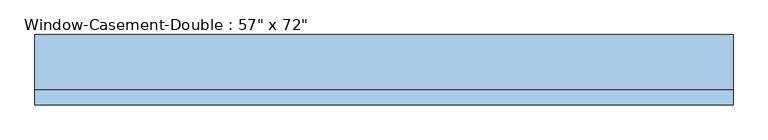
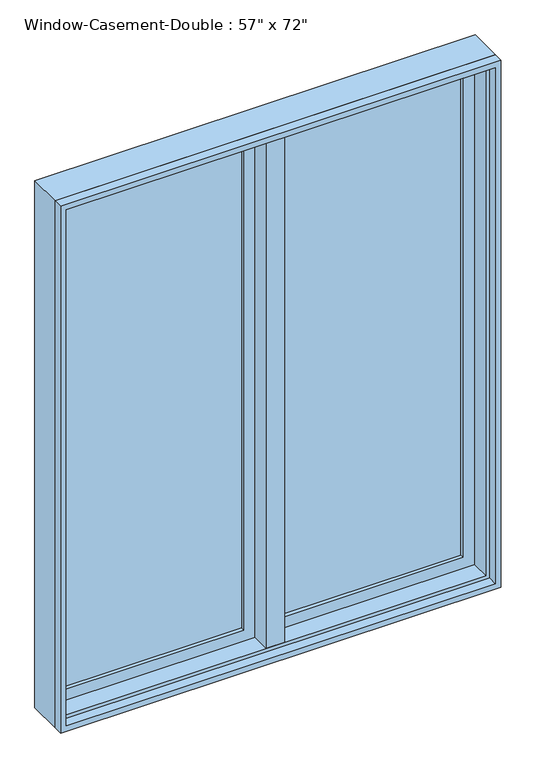
"""IFC4 building model written with IfcOpenShell, lengths in millimetres: window geometry."""

from ifc_helpers import new_model, si_unit, frame, origin, place, context, project, spatial, polyline, outline, extrude, faceted_brep, source, transform, mapped, element, save


def window_51a0d18f(model_context):
    return source(origin(), model_context, "Body", "SolidModel", [
        faceted_brep([(9.525, 82.55, 2730.5), (-9.525, 82.55, 2730.5), (-9.525, 31.75, 2730.5), (9.525, 31.75, 2730.5), (9.525, 82.55, 927.1), (9.525, 31.75, 927.1), (-9.525, 31.75, 927.1), (-9.525, 82.55, 927.1), (-9.525, 31.75, 946.15), (-9.525, 31.75, 2711.45), (-30.1625, 31.75, 946.15), (-30.1625, 31.75, 2711.45), (-30.1625, -31.75, 946.15), (-30.1625, -31.75, 2711.45), (30.1625, -31.75, 946.15), (30.1625, -31.75, 2711.45), (30.1625, 31.75, 946.15), (30.1625, 31.75, 2711.45), (9.525, 31.75, 946.15), (9.525, 31.75, 2711.45)], [[[0, 1, 2, 3]], [[4, 5, 6, 7]], [[1, 0, 4, 7]], [[2, 1, 7, 6, 8, 9]], [[9, 8, 10, 11]], [[11, 10, 12, 13]], [[13, 12, 14, 15]], [[15, 14, 16, 17]], [[17, 16, 18, 19]], [[0, 3, 19, 18, 5, 4]], [[18, 8, 6, 5]], [[9, 19, 3, 2]], [[8, 18, 16, 14, 12, 10]], [[19, 9, 11, 13, 15, 17]]]),
        extrude(outline(polyline([(-66.675, 63.5), (-66.675, 57.15), (-654.05, 57.15), (-654.05, 63.5), (-66.675, 63.5)])), frame((0.0, 0.0, 984.25), z_axis=(0.0, 0.0, 1.0), x_axis=(1.0, 0.0, 0.0)), (0.0, 0.0, 1.0), 1689.1),
        extrude(outline(polyline([(-654.05, 44.45), (-654.05, 50.8), (-66.675, 50.8), (-66.675, 44.45), (-654.05, 44.45)])), frame((0.0, 0.0, 984.25), z_axis=(0.0, 0.0, 1.0), x_axis=(1.0, 0.0, 0.0)), (0.0, 0.0, 1.0), 1689.1),
        extrude(outline(polyline([(654.05, 63.5), (654.05, 57.15), (66.675, 57.15), (66.675, 63.5), (654.05, 63.5)])), frame((0.0, 0.0, 984.25), z_axis=(0.0, 0.0, 1.0), x_axis=(1.0, 0.0, 0.0)), (0.0, 0.0, 1.0), 1689.1),
        extrude(outline(polyline([(66.675, 44.45), (66.675, 50.8), (654.05, 50.8), (654.05, 44.45), (66.675, 44.45)])), frame((0.0, 0.0, 984.25), z_axis=(0.0, 0.0, 1.0), x_axis=(1.0, 0.0, 0.0)), (0.0, 0.0, 1.0), 1689.1),
        extrude(outline(polyline([(2730.5, -711.2), (927.1, -711.2), (927.1, -9.525), (2730.5, -9.525), (2730.5, -711.2)]), holes=[polyline([(2673.35, -66.675), (984.25, -66.675), (984.25, -654.05), (2673.35, -654.05), (2673.35, -66.675)])]), frame((0.0, 31.75, 0.0), z_axis=(0.0, 1.0, 0.0), x_axis=(0.0, 0.0, 1.0)), (0.0, 0.0, 1.0), 44.45),
        extrude(outline(polyline([(927.1, 711.2), (2730.5, 711.2), (2730.5, 9.525), (927.1, 9.525), (927.1, 711.2)]), holes=[polyline([(984.25, 66.675), (2673.35, 66.675), (2673.35, 654.05), (984.25, 654.05), (984.25, 66.675)])]), frame((0.0, 31.75, 0.0), z_axis=(0.0, 1.0, 0.0), x_axis=(0.0, 0.0, 1.0)), (0.0, 0.0, 1.0), 44.45),
        extrude(outline(polyline([(2743.2, -723.9), (914.4, -723.9), (914.4, 723.9), (2743.2, 723.9), (2743.2, -723.9)]), holes=[polyline([(2724.15, 704.85), (933.45, 704.85), (933.45, -704.85), (2724.15, -704.85), (2724.15, 704.85)])]), frame((0.0, -63.5, 0.0), z_axis=(0.0, 1.0, 0.0), x_axis=(0.0, 0.0, 1.0)), (0.0, 0.0, 1.0), 31.75),
        faceted_brep([(692.15, 31.75, 2711.45), (692.15, -31.75, 2711.45), (-692.15, -31.75, 2711.45), (-692.15, 31.75, 2711.45), (711.2, 82.55, 2730.5), (711.2, 31.75, 2730.5), (-711.2, 31.75, 2730.5), (-711.2, 82.55, 2730.5), (723.9, -31.75, 2743.2), (723.9, 82.55, 2743.2), (-723.9, 82.55, 2743.2), (-723.9, -31.75, 2743.2), (-692.15, -31.75, 946.15), (-692.15, 31.75, 946.15), (-711.2, 31.75, 927.1), (-711.2, 82.55, 927.1), (-723.9, 82.55, 914.4), (-723.9, -31.75, 914.4), (692.15, -31.75, 946.15), (692.15, 31.75, 946.15), (711.2, 31.75, 927.1), (711.2, 82.55, 927.1), (723.9, 82.55, 914.4), (723.9, -31.75, 914.4)], [[[0, 1, 2, 3]], [[4, 5, 6, 7]], [[8, 9, 10, 11]], [[3, 2, 12, 13]], [[7, 6, 14, 15]], [[11, 10, 16, 17]], [[13, 12, 18, 19]], [[15, 14, 20, 21]], [[17, 16, 22, 23]], [[11, 17, 23, 8], [1, 18, 12, 2]], [[19, 18, 1, 0]], [[5, 20, 14, 6], [3, 13, 19, 0]], [[21, 20, 5, 4]], [[23, 22, 9, 8]], [[9, 22, 16, 10], [7, 15, 21, 4]]]),
    ])


if __name__ == "__main__":
    model = new_model("IFC4")
    model_context = context("Model", 3, world=origin())
    ifc_project = project(units=[si_unit("LENGTHUNIT", "METRE", prefix="MILLI")], contexts=[model_context])
    site = spatial("IfcSite", under=ifc_project)
    building = spatial("IfcBuilding", under=site)
    placement = place(None, origin())
    window_shape = window_51a0d18f(model_context)
    element("IfcWindow", 1, ObjectType="Window-Casement-Double : 57\" x 72\"", at=placement, inside=building, context=model_context, shape_type="MappedRepresentation", body=[
        mapped(window_shape, transform((0.0, 0.0, 0.0), x_axis=(1.0, 0.0, 0.0), y_axis=(0.0, 1.0, 0.0), z_axis=(0.0, 0.0, 1.0))),
    ])
    save(model, "model.ifc")

# Revit data of these elements
# Type "Window-Casement-Double : 57\" x 72\""
#   Type Mark = "17"
#   Fire Rating = "0.5h"
#   Assembly Code = "B2020100"
#   Analytic Construction = "Double glazing - domestic"
#   Frame Extension [instance default] = 0' - 0 1/4"
#   Window Inset [instance default] = 0' - 0"
#   Wall Thickness [instance default] = 0' - 6"
#   Interior Wall Closure [instance default] = 0' - 2 1/4"
#   Half Width = 2' - 4 1/2"
#   Visual Light Transmittance = 0.81
#   Thermal Resistance (R) = 1.8146 (h·ft²·°F)/BTU
#   Solar Heat Gain Coefficient = 0.76
#   Rough Width = 4' - 9 1/2"
#   Rough Height = 6' - 0 1/2"
#   Height = 6' - 0"
#   Heat Transfer Coefficient (U) = 0.5511 BTU/(h·ft²·°F)
#   Exterior Wall Closure [instance default] = 0' - 1 1/4"
#   Extension Jamb [instance default] = 0' - 2 1/4"
#   Default Sill Height = 3' - 0"
#   Width = 4' - 9"
#   Define Thermal Properties by = 0
#   Muntin Visibility = yes
#   Interior Trim Visibility [instance default] = yes
#   Exterior Trim Visibility [instance default] = yes
#   Extension Jamb Visibility [instance default] = yes
#   Interior Trim Material = Wood - Stained
#   Muntin Pattern = Muntin Pattern_2x2 : Muntin Pattern_2x2
#   Interior Trim = Trim-Window-Interior-Flat : Picture Frame
#   Interior Frame Material = Wood - Stained
#   Glass Panel Material = Glass
#   Exterior Trim Material = Clad - White
#   Exterior Trim = Trim-Window-Exterior-Flat : with Sill
#   Exterior Frame Material = Clad - White
#   Wall Closure = (empty or 0)
# Element 1 (IfcWindow, "Window-Casement-Double : 57\" x 72\"")
#   Wall Thickness = 0' - 5"
#   Extension Jamb = 0' - 1 1/4"
#   Materials on its faces: "Wood - Stained", "Glass", "Clad - White"
# Materials
#   "Wood - Stained": class "Wood", colour RGB 224 178 126, transparency 0, Cost = 0
#   "Glass": class "Glass", colour RGB 0 128 192, transparency 0.75, Description = "Soda Lime Glass", Cost = 0
#   "Clad - White": class "Wood", colour RGB 242 242 238, transparency 0, Cost = 0
